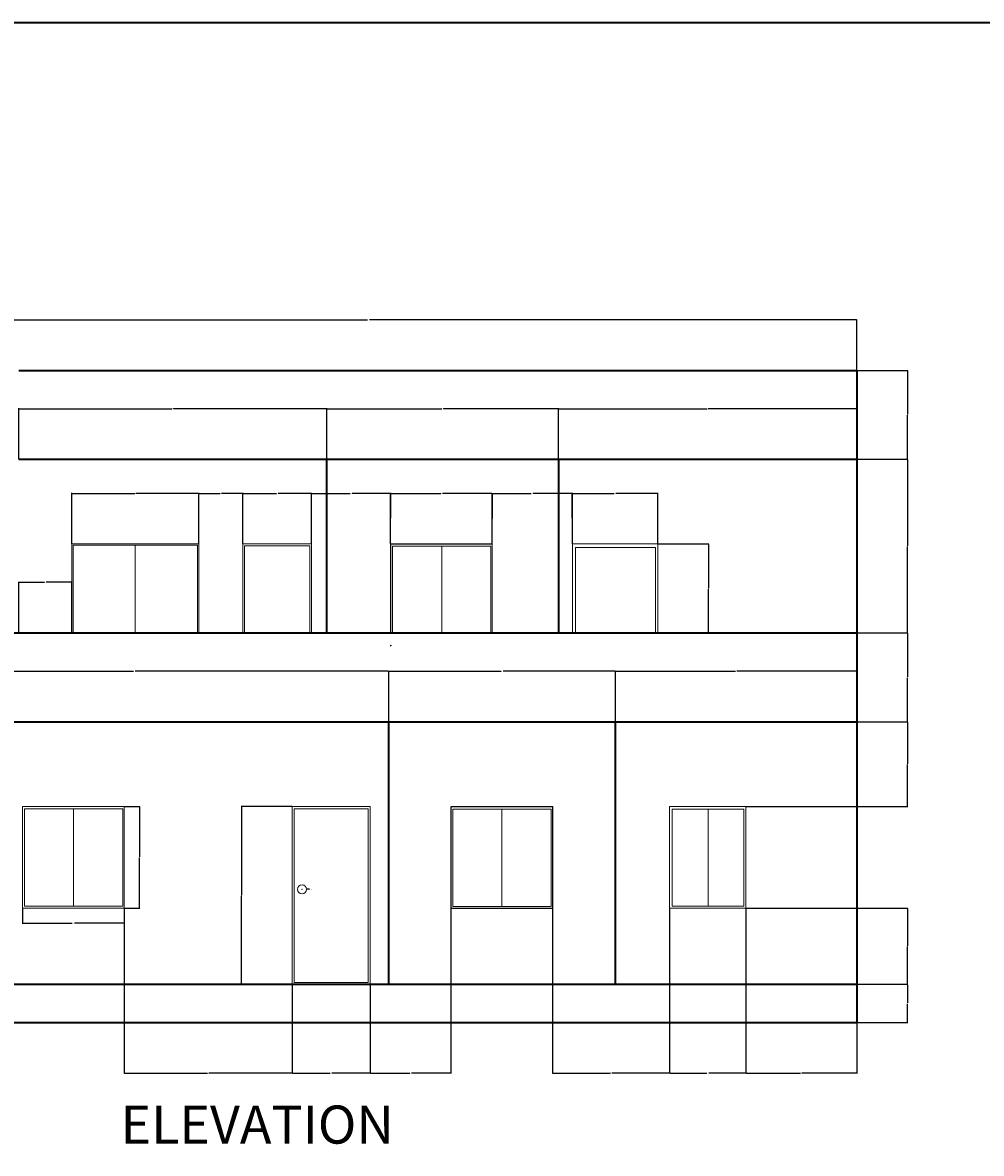
# Model space of a CAD drawing. Units: inches. Extents: x 2067 to 3463, y 1605 to 2723.
# Tile 7 of 10: x 2312 to 2765, y 2189 to 2723. Entities that reach past the tile are written whole.
import ezdxf

# ---------------------------------------------------------------- set-up
doc = ezdxf.new("R2010")
doc.units = ezdxf.units.IN
for name, color, linetype, lineweight in [('A-ANNO-DIMS', 2, 'Continuous', 18), ('A-ANNO-TEXT', 7, 'Continuous', 35), ('A-ANNO-TTLB', 7, 'Continuous', 35), ('A-ELEV', 7, 'Continuous', 35), ('A-ELEV-DOOR', 3, 'Continuous', 18), ('A-ELEV-GLAZ', 4, 'Continuous', 18)]:
    doc.layers.add(name, color=color, linetype=linetype, lineweight=lineweight)
doc.styles.get("Standard").update_dxf_attribs({"font": 'arial.ttf'})
doc.dimstyles.get("Standard").update_dxf_attribs({"dimtxt": 0.18, "dimasz": 0.18, "dimexe": 0.18, "dimexo": 0.0625, "dimgap": 0.09, "dimtad": 0, "dimtih": 1, "dimtoh": 1, "dimdec": 4, "dimzin": 0, "dimdsep": 46, "dimtxsty": 'Standard', "dimcen": 0.09, "dimadec": 0, "dimazin": 0, "dimtfac": 1, "dimtdec": 4, "dimtofl": 0, "dimtmove": 0, "dimatfit": 3, "dimfxl": 1, "dimtolj": 1, "dimtzin": 0, "dimarcsym": 0})

# ---------------------------------------------------------------- blocks, each defined once
blk = doc.blocks.new('WIN-ELEV-48X48')
for p, q in [((0, 48), (0, 0)), ((0, 48), (48, 48)), ((24.11, 0.97), (24.11, 46.96)), ((48, 48), (48, 0)), ((0, 0), (48, 0))]:
    blk.add_line(p, q)
blk.add_lwpolyline([(0.84, 46.96), (47.38, 46.96), (47.38, 0.97), (0.84, 0.97)], close=True)
blk = doc.blocks.new('*D26')
at = {"layer": 'A-ANNO-DIMS', "color": 0, "lineweight": -2, "transparency": 16777216}
for p, q in [((2360.32, 2352.37), (2367.64, 2352.37)), ((2367.46, 2352.19), (2367.46, 2328.55)), ((2367.46, 2304.55), (2367.46, 2328.18)), ((2360.32, 2304.37), (2367.64, 2304.37))]:
    blk.add_line(p, q, dxfattribs=at)
at = {"layer": 'A-ANNO-DIMS', "color": 0, "transparency": 16777216}
for points in [[(2367.43, 2352.19), (2367.49, 2352.19), (2367.46, 2352.37)], [(2367.43, 2304.55), (2367.49, 2304.55), (2367.46, 2304.37)]]:
    blk.add_solid(points, dxfattribs=at)
at = {"layer": 'Defpoints', "color": 0, "transparency": 16777216}
for p in [(2360.26, 2352.37), (2367.46, 2352.37), (2360.26, 2304.37)]:
    blk.add_point(p, dxfattribs=at)
at = {"layer": 'A-ANNO-DIMS', "color": 0, "transparency": 16777216, "insert": (2367.46, 2328.37), "char_height": 0.18, "attachment_point": 5}
blk.add_mtext('\\A1;WINDOW 48 TYP.', dxfattribs=at)
blk = doc.blocks.new('*D27')
at = {"layer": 'A-ANNO-DIMS', "color": 0, "lineweight": -2, "transparency": 16777216}
for p, q in [((2312.26, 2304.3), (2312.26, 2296.99)), ((2360.26, 2304.3), (2360.26, 2296.99)), ((2312.44, 2297.17), (2335.73, 2297.17)), ((2360.08, 2297.17), (2336.79, 2297.17))]:
    blk.add_line(p, q, dxfattribs=at)
at = {"layer": 'A-ANNO-DIMS', "color": 0, "transparency": 16777216}
for points in [[(2312.44, 2297.2), (2312.44, 2297.14), (2312.26, 2297.17)], [(2360.08, 2297.2), (2360.08, 2297.14), (2360.26, 2297.17)]]:
    blk.add_solid(points, dxfattribs=at)
at = {"layer": 'Defpoints', "color": 0, "transparency": 16777216}
for p in [(2312.26, 2304.37), (2360.26, 2304.37), (2360.26, 2297.17)]:
    blk.add_point(p, dxfattribs=at)
at = {"layer": 'A-ANNO-DIMS', "color": 0, "transparency": 16777216, "insert": (2336.26, 2297.17), "char_height": 0.18, "attachment_point": 5}
blk.add_mtext('\\A1;48 TYP.', dxfattribs=at)
blk = doc.blocks.new('*D69')
at = {"layer": 'A-ANNO-DIMS', "color": 0, "lineweight": -2, "transparency": 16777216}
for p, q in [((2244.95, 2434.43), (2244.95, 2582.45)), ((2245.13, 2582.27), (2475.3, 2582.27)), ((2706.27, 2582.27), (2476.1, 2582.27)), ((2706.45, 2558.43), (2706.45, 2582.45))]:
    blk.add_line(p, q, dxfattribs=at)
at = {"layer": 'A-ANNO-DIMS', "color": 0, "transparency": 16777216}
for points in [[(2245.13, 2582.3), (2245.13, 2582.24), (2244.95, 2582.27)], [(2706.27, 2582.3), (2706.27, 2582.24), (2706.45, 2582.27)]]:
    blk.add_solid(points, dxfattribs=at)
at = {"layer": 'Defpoints', "color": 0, "transparency": 16777216}
for p in [(2706.45, 2582.27), (2706.45, 2558.37), (2244.95, 2434.37)]:
    blk.add_point(p, dxfattribs=at)
at = {"layer": 'A-ANNO-DIMS', "color": 0, "transparency": 16777216, "insert": (2475.7, 2582.27), "char_height": 0.18, "attachment_point": 5}
blk.add_mtext('\\A1;461.5', dxfattribs=at)
blk = doc.blocks.new('*D71')
at = {"layer": 'A-ANNO-DIMS', "color": 0, "lineweight": -2, "transparency": 16777216}
for p, q in [((2706.51, 2268.37), (2730.53, 2268.37)), ((2730.35, 2268.19), (2730.35, 2259.55)), ((2730.35, 2250.55), (2730.35, 2259.18)), ((2706.51, 2250.37), (2730.53, 2250.37))]:
    blk.add_line(p, q, dxfattribs=at)
at = {"layer": 'A-ANNO-DIMS', "color": 0, "transparency": 16777216}
for points in [[(2730.32, 2268.19), (2730.38, 2268.19), (2730.35, 2268.37)], [(2730.32, 2250.55), (2730.38, 2250.55), (2730.35, 2250.37)]]:
    blk.add_solid(points, dxfattribs=at)
at = {"layer": 'Defpoints', "color": 0, "transparency": 16777216}
for p in [(2706.45, 2268.37), (2730.35, 2268.37), (2706.45, 2250.37)]:
    blk.add_point(p, dxfattribs=at)
at = {"layer": 'A-ANNO-DIMS', "color": 0, "transparency": 16777216, "insert": (2730.35, 2259.37), "char_height": 0.18, "attachment_point": 5}
blk.add_mtext('\\A1;18', dxfattribs=at)
blk = doc.blocks.new('*D72')
at = {"layer": 'A-ANNO-DIMS', "color": 0, "lineweight": -2, "transparency": 16777216}
for p, q in [((2654.01, 2304.37), (2730.53, 2304.37)), ((2730.35, 2304.19), (2730.35, 2286.55)), ((2730.35, 2268.55), (2730.35, 2286.18)), ((2706.51, 2268.37), (2730.53, 2268.37))]:
    blk.add_line(p, q, dxfattribs=at)
at = {"layer": 'A-ANNO-DIMS', "color": 0, "transparency": 16777216}
for points in [[(2730.32, 2304.19), (2730.38, 2304.19), (2730.35, 2304.37)], [(2730.32, 2268.55), (2730.38, 2268.55), (2730.35, 2268.37)]]:
    blk.add_solid(points, dxfattribs=at)
at = {"layer": 'Defpoints', "color": 0, "transparency": 16777216}
for p in [(2653.95, 2304.37), (2730.35, 2304.37), (2706.45, 2268.37)]:
    blk.add_point(p, dxfattribs=at)
at = {"layer": 'A-ANNO-DIMS', "color": 0, "transparency": 16777216, "insert": (2730.35, 2286.37), "char_height": 0.18, "attachment_point": 5}
blk.add_mtext('\\A1;36', dxfattribs=at)
blk = doc.blocks.new('*D73')
at = {"layer": 'A-ANNO-DIMS', "color": 0, "lineweight": -2, "transparency": 16777216}
for p, q in [((2706.51, 2392.37), (2730.53, 2392.37)), ((2730.35, 2392.19), (2730.35, 2372.55)), ((2730.35, 2352.55), (2730.35, 2372.18)), ((2654.01, 2352.37), (2730.53, 2352.37))]:
    blk.add_line(p, q, dxfattribs=at)
at = {"layer": 'A-ANNO-DIMS', "color": 0, "transparency": 16777216}
for points in [[(2730.32, 2392.19), (2730.38, 2392.19), (2730.35, 2392.37)], [(2730.32, 2352.55), (2730.38, 2352.55), (2730.35, 2352.37)]]:
    blk.add_solid(points, dxfattribs=at)
at = {"layer": 'Defpoints', "color": 0, "transparency": 16777216}
for p in [(2706.45, 2392.37), (2730.35, 2392.37), (2653.95, 2352.37)]:
    blk.add_point(p, dxfattribs=at)
at = {"layer": 'A-ANNO-DIMS', "color": 0, "transparency": 16777216, "insert": (2730.35, 2372.37), "char_height": 0.18, "attachment_point": 5}
blk.add_mtext('\\A1;40', dxfattribs=at)
blk = doc.blocks.new('*D74')
at = {"layer": 'A-ANNO-DIMS', "color": 0, "lineweight": -2, "transparency": 16777216}
for p, q in [((2706.51, 2434.37), (2730.53, 2434.37)), ((2730.35, 2434.19), (2730.35, 2413.55)), ((2730.35, 2392.55), (2730.35, 2413.19)), ((2706.51, 2392.37), (2730.53, 2392.37))]:
    blk.add_line(p, q, dxfattribs=at)
at = {"layer": 'A-ANNO-DIMS', "color": 0, "transparency": 16777216}
for points in [[(2730.32, 2434.19), (2730.38, 2434.19), (2730.35, 2434.37)], [(2730.32, 2392.55), (2730.38, 2392.55), (2730.35, 2392.37)]]:
    blk.add_solid(points, dxfattribs=at)
at = {"layer": 'Defpoints', "color": 0, "transparency": 16777216}
for p in [(2706.45, 2434.37), (2730.35, 2434.37), (2706.45, 2392.37)]:
    blk.add_point(p, dxfattribs=at)
at = {"layer": 'A-ANNO-DIMS', "color": 0, "transparency": 16777216, "insert": (2730.35, 2413.37), "char_height": 0.18, "attachment_point": 5}
blk.add_mtext('\\A1;42', dxfattribs=at)
blk = doc.blocks.new('*D75')
at = {"layer": 'A-ANNO-DIMS', "color": 0, "lineweight": -2, "transparency": 16777216}
for p, q in [((2706.51, 2516.37), (2730.53, 2516.37)), ((2730.35, 2516.19), (2730.35, 2475.55)), ((2730.35, 2434.55), (2730.35, 2475.18)), ((2706.51, 2434.37), (2730.53, 2434.37))]:
    blk.add_line(p, q, dxfattribs=at)
at = {"layer": 'A-ANNO-DIMS', "color": 0, "transparency": 16777216}
for points in [[(2730.32, 2516.19), (2730.38, 2516.19), (2730.35, 2516.37)], [(2730.32, 2434.55), (2730.38, 2434.55), (2730.35, 2434.37)]]:
    blk.add_solid(points, dxfattribs=at)
at = {"layer": 'Defpoints', "color": 0, "transparency": 16777216}
for p in [(2706.45, 2516.37), (2730.35, 2516.37), (2706.45, 2434.37)]:
    blk.add_point(p, dxfattribs=at)
at = {"layer": 'A-ANNO-DIMS', "color": 0, "transparency": 16777216, "insert": (2730.35, 2475.37), "char_height": 0.18, "attachment_point": 5}
blk.add_mtext('\\A1;82', dxfattribs=at)
blk = doc.blocks.new('*D76')
at = {"layer": 'A-ANNO-DIMS', "color": 0, "lineweight": -2, "transparency": 16777216}
for p, q in [((2706.51, 2558.37), (2730.53, 2558.37)), ((2730.35, 2558.19), (2730.35, 2537.55)), ((2730.35, 2516.55), (2730.35, 2537.19)), ((2706.51, 2516.37), (2730.53, 2516.37))]:
    blk.add_line(p, q, dxfattribs=at)
at = {"layer": 'A-ANNO-DIMS', "color": 0, "transparency": 16777216}
for points in [[(2730.32, 2558.19), (2730.38, 2558.19), (2730.35, 2558.37)], [(2730.32, 2516.55), (2730.38, 2516.55), (2730.35, 2516.37)]]:
    blk.add_solid(points, dxfattribs=at)
at = {"layer": 'Defpoints', "color": 0, "transparency": 16777216}
for p in [(2706.45, 2558.37), (2730.35, 2558.37), (2706.45, 2516.37)]:
    blk.add_point(p, dxfattribs=at)
at = {"layer": 'A-ANNO-DIMS', "color": 0, "transparency": 16777216, "insert": (2730.35, 2537.37), "char_height": 0.18, "attachment_point": 5}
blk.add_mtext('\\A1;42', dxfattribs=at)
blk = doc.blocks.new('*D78')
at = {"layer": 'A-ANNO-DIMS', "color": 0, "lineweight": -2, "transparency": 16777216}
for p, q in [((2310.45, 2516.43), (2310.45, 2540.45)), ((2310.63, 2540.27), (2382.81, 2540.27)), ((2455.77, 2540.27), (2383.58, 2540.27)), ((2455.95, 2516.43), (2455.95, 2540.45))]:
    blk.add_line(p, q, dxfattribs=at)
at = {"layer": 'A-ANNO-DIMS', "color": 0, "transparency": 16777216}
for points in [[(2310.63, 2540.3), (2310.63, 2540.24), (2310.45, 2540.27)], [(2455.77, 2540.3), (2455.77, 2540.24), (2455.95, 2540.27)]]:
    blk.add_solid(points, dxfattribs=at)
at = {"layer": 'Defpoints', "color": 0, "transparency": 16777216}
for p in [(2455.95, 2540.27), (2310.45, 2516.37), (2455.95, 2516.37)]:
    blk.add_point(p, dxfattribs=at)
at = {"layer": 'A-ANNO-DIMS', "color": 0, "transparency": 16777216, "insert": (2383.2, 2540.27), "char_height": 0.18, "attachment_point": 5}
blk.add_mtext('\\A1;145.5', dxfattribs=at)
blk = doc.blocks.new('*D79')
at = {"layer": 'A-ANNO-DIMS', "color": 0, "lineweight": -2, "transparency": 16777216}
for p, q in [((2455.95, 2516.43), (2455.95, 2540.45)), ((2456.13, 2540.27), (2510.31, 2540.27)), ((2565.27, 2540.27), (2511.08, 2540.27)), ((2565.45, 2516.43), (2565.45, 2540.45))]:
    blk.add_line(p, q, dxfattribs=at)
at = {"layer": 'A-ANNO-DIMS', "color": 0, "transparency": 16777216}
for points in [[(2456.13, 2540.3), (2456.13, 2540.24), (2455.95, 2540.27)], [(2565.27, 2540.3), (2565.27, 2540.24), (2565.45, 2540.27)]]:
    blk.add_solid(points, dxfattribs=at)
at = {"layer": 'Defpoints', "color": 0, "transparency": 16777216}
for p in [(2565.45, 2540.27), (2455.95, 2516.37), (2565.45, 2516.37)]:
    blk.add_point(p, dxfattribs=at)
at = {"layer": 'A-ANNO-DIMS', "color": 0, "transparency": 16777216, "insert": (2510.7, 2540.27), "char_height": 0.18, "attachment_point": 5}
blk.add_mtext('\\A1;109.5', dxfattribs=at)
blk = doc.blocks.new('*D80')
at = {"layer": 'A-ANNO-DIMS', "color": 0, "lineweight": -2, "transparency": 16777216}
for p, q in [((2565.45, 2516.43), (2565.45, 2540.45)), ((2565.63, 2540.27), (2635.68, 2540.27)), ((2706.27, 2540.27), (2636.21, 2540.27)), ((2706.45, 2516.43), (2706.45, 2540.45))]:
    blk.add_line(p, q, dxfattribs=at)
at = {"layer": 'A-ANNO-DIMS', "color": 0, "transparency": 16777216}
for points in [[(2565.63, 2540.3), (2565.63, 2540.24), (2565.45, 2540.27)], [(2706.27, 2540.3), (2706.27, 2540.24), (2706.45, 2540.27)]]:
    blk.add_solid(points, dxfattribs=at)
at = {"layer": 'Defpoints', "color": 0, "transparency": 16777216}
for p in [(2706.45, 2540.27), (2565.45, 2516.37), (2706.45, 2516.37)]:
    blk.add_point(p, dxfattribs=at)
at = {"layer": 'A-ANNO-DIMS', "color": 0, "transparency": 16777216, "insert": (2635.95, 2540.27), "char_height": 0.18, "attachment_point": 5}
blk.add_mtext('\\A1;141', dxfattribs=at)
blk = doc.blocks.new('*D81')
at = {"layer": 'A-ANNO-DIMS', "color": 0, "lineweight": -2, "transparency": 16777216}
for p, q in [((2310.45, 2434.43), (2310.45, 2458.45)), ((2310.63, 2458.27), (2322.63, 2458.27)), ((2335.38, 2458.27), (2323.38, 2458.27)), ((2335.56, 2434.43), (2335.56, 2458.45))]:
    blk.add_line(p, q, dxfattribs=at)
at = {"layer": 'A-ANNO-DIMS', "color": 0, "transparency": 16777216}
for points in [[(2310.63, 2458.3), (2310.63, 2458.24), (2310.45, 2458.27)], [(2335.38, 2458.3), (2335.38, 2458.24), (2335.56, 2458.27)]]:
    blk.add_solid(points, dxfattribs=at)
at = {"layer": 'Defpoints', "color": 0, "transparency": 16777216}
for p in [(2335.56, 2458.27), (2310.45, 2434.37), (2335.56, 2434.37)]:
    blk.add_point(p, dxfattribs=at)
at = {"layer": 'A-ANNO-DIMS', "color": 0, "transparency": 16777216, "insert": (2323, 2458.27), "char_height": 0.18, "attachment_point": 5}
blk.add_mtext('\\A1;25.11', dxfattribs=at)
blk = doc.blocks.new('*D82')
at = {"layer": 'A-ANNO-DIMS', "color": 0, "lineweight": -2, "transparency": 16777216}
for p, q in [((2335.56, 2476.43), (2335.56, 2500.45)), ((2335.74, 2500.27), (2365.34, 2500.27)), ((2395.38, 2500.27), (2365.78, 2500.27)), ((2395.56, 2476.43), (2395.56, 2500.45))]:
    blk.add_line(p, q, dxfattribs=at)
at = {"layer": 'A-ANNO-DIMS', "color": 0, "transparency": 16777216}
for points in [[(2335.74, 2500.3), (2335.74, 2500.24), (2335.56, 2500.27)], [(2395.38, 2500.3), (2395.38, 2500.24), (2395.56, 2500.27)]]:
    blk.add_solid(points, dxfattribs=at)
at = {"layer": 'Defpoints', "color": 0, "transparency": 16777216}
for p in [(2395.56, 2500.27), (2335.56, 2476.37), (2395.56, 2476.37)]:
    blk.add_point(p, dxfattribs=at)
at = {"layer": 'A-ANNO-DIMS', "color": 0, "transparency": 16777216, "insert": (2365.56, 2500.27), "char_height": 0.18, "attachment_point": 5}
blk.add_mtext('\\A1;60', dxfattribs=at)
blk = doc.blocks.new('*D83')
at = {"layer": 'A-ANNO-DIMS', "color": 0, "lineweight": -2, "transparency": 16777216}
for p, q in [((2395.56, 2476.43), (2395.56, 2500.45)), ((2395.74, 2500.27), (2405.63, 2500.27)), ((2416.18, 2500.27), (2406.28, 2500.27)), ((2416.36, 2476.43), (2416.36, 2500.45))]:
    blk.add_line(p, q, dxfattribs=at)
at = {"layer": 'A-ANNO-DIMS', "color": 0, "transparency": 16777216}
for points in [[(2395.74, 2500.3), (2395.74, 2500.24), (2395.56, 2500.27)], [(2416.18, 2500.3), (2416.18, 2500.24), (2416.36, 2500.27)]]:
    blk.add_solid(points, dxfattribs=at)
at = {"layer": 'Defpoints', "color": 0, "transparency": 16777216}
for p in [(2416.36, 2500.27), (2395.56, 2476.37), (2416.36, 2476.37)]:
    blk.add_point(p, dxfattribs=at)
at = {"layer": 'A-ANNO-DIMS', "color": 0, "transparency": 16777216, "insert": (2405.96, 2500.27), "char_height": 0.18, "attachment_point": 5}
blk.add_mtext('\\A1;20.8', dxfattribs=at)
blk = doc.blocks.new('*D84')
at = {"layer": 'A-ANNO-DIMS', "color": 0, "lineweight": -2, "transparency": 16777216}
for p, q in [((2416.36, 2476.43), (2416.36, 2500.45)), ((2416.54, 2500.27), (2432.18, 2500.27)), ((2448.62, 2500.27), (2432.97, 2500.27)), ((2448.8, 2476.43), (2448.8, 2500.45))]:
    blk.add_line(p, q, dxfattribs=at)
at = {"layer": 'A-ANNO-DIMS', "color": 0, "transparency": 16777216}
for points in [[(2416.54, 2500.3), (2416.54, 2500.24), (2416.36, 2500.27)], [(2448.62, 2500.3), (2448.62, 2500.24), (2448.8, 2500.27)]]:
    blk.add_solid(points, dxfattribs=at)
at = {"layer": 'Defpoints', "color": 0, "transparency": 16777216}
for p in [(2448.8, 2500.27), (2416.36, 2476.37), (2448.8, 2476.37)]:
    blk.add_point(p, dxfattribs=at)
at = {"layer": 'A-ANNO-DIMS', "color": 0, "transparency": 16777216, "insert": (2432.58, 2500.27), "char_height": 0.18, "attachment_point": 5}
blk.add_mtext('\\A1;32.44', dxfattribs=at)
blk = doc.blocks.new('*D85')
at = {"layer": 'A-ANNO-DIMS', "color": 0, "lineweight": -2, "transparency": 16777216}
for p, q in [((2448.8, 2476.43), (2448.8, 2500.45)), ((2448.98, 2500.27), (2467.02, 2500.27)), ((2485.98, 2500.27), (2467.94, 2500.27)), ((2486.16, 2476.43), (2486.16, 2500.45))]:
    blk.add_line(p, q, dxfattribs=at)
at = {"layer": 'A-ANNO-DIMS', "color": 0, "transparency": 16777216}
for points in [[(2448.98, 2500.3), (2448.98, 2500.24), (2448.8, 2500.27)], [(2485.98, 2500.3), (2485.98, 2500.24), (2486.16, 2500.27)]]:
    blk.add_solid(points, dxfattribs=at)
at = {"layer": 'Defpoints', "color": 0, "transparency": 16777216}
for p in [(2486.16, 2500.27), (2448.8, 2476.37), (2486.16, 2476.37)]:
    blk.add_point(p, dxfattribs=at)
at = {"layer": 'A-ANNO-DIMS', "color": 0, "transparency": 16777216, "insert": (2467.48, 2500.27), "char_height": 0.18, "attachment_point": 5}
blk.add_mtext('\\A1;37.365', dxfattribs=at)
blk = doc.blocks.new('*D86')
at = {"layer": 'A-ANNO-DIMS', "color": 0, "lineweight": -2, "transparency": 16777216}
for p, q in [((2486.16, 2476.43), (2486.2, 2500.45)), ((2486.38, 2500.27), (2509.81, 2500.23)), ((2534.04, 2500.19), (2510.61, 2500.23)), ((2534.18, 2476.35), (2534.22, 2500.37))]:
    blk.add_line(p, q, dxfattribs=at)
at = {"layer": 'A-ANNO-DIMS', "color": 0, "transparency": 16777216}
for points in [[(2486.38, 2500.3), (2486.38, 2500.24), (2486.2, 2500.27)], [(2534.04, 2500.22), (2534.04, 2500.16), (2534.22, 2500.19)]]:
    blk.add_solid(points, dxfattribs=at)
at = {"layer": 'Defpoints', "color": 0, "transparency": 16777216}
for p in [(2534.22, 2500.19), (2486.16, 2476.37), (2534.18, 2476.29)]:
    blk.add_point(p, dxfattribs=at)
at = {"layer": 'A-ANNO-DIMS', "color": 0, "transparency": 16777216, "insert": (2510.21, 2500.23), "char_height": 0.18, "attachment_point": 5}
blk.add_mtext('\\A1;48.02', dxfattribs=at)
blk = doc.blocks.new('*D87')
at = {"layer": 'A-ANNO-DIMS', "color": 0, "lineweight": -2, "transparency": 16777216}
for p, q in [((2534.18, 2476.35), (2534.14, 2500.37)), ((2534.32, 2500.19), (2552.59, 2500.23)), ((2571.8, 2500.27), (2553.52, 2500.23)), ((2572.03, 2476.43), (2571.98, 2500.45))]:
    blk.add_line(p, q, dxfattribs=at)
at = {"layer": 'A-ANNO-DIMS', "color": 0, "transparency": 16777216}
for points in [[(2534.32, 2500.22), (2534.32, 2500.16), (2534.14, 2500.19)], [(2571.8, 2500.3), (2571.8, 2500.24), (2571.98, 2500.27)]]:
    blk.add_solid(points, dxfattribs=at)
at = {"layer": 'Defpoints', "color": 0, "transparency": 16777216}
for p in [(2571.98, 2500.27), (2534.18, 2476.29), (2572.03, 2476.37)]:
    blk.add_point(p, dxfattribs=at)
at = {"layer": 'A-ANNO-DIMS', "color": 0, "transparency": 16777216, "insert": (2553.06, 2500.23), "char_height": 0.18, "attachment_point": 5}
blk.add_mtext('\\A1;37.844', dxfattribs=at)
blk = doc.blocks.new('*D88')
at = {"layer": 'A-ANNO-DIMS', "color": 0, "lineweight": -2, "transparency": 16777216}
for p, q in [((2572.03, 2476.43), (2572.03, 2500.45)), ((2572.21, 2500.27), (2591.84, 2500.27)), ((2612.27, 2500.27), (2592.63, 2500.27)), ((2612.45, 2476.43), (2612.45, 2500.45))]:
    blk.add_line(p, q, dxfattribs=at)
at = {"layer": 'A-ANNO-DIMS', "color": 0, "transparency": 16777216}
for points in [[(2572.21, 2500.3), (2572.21, 2500.24), (2572.03, 2500.27)], [(2612.27, 2500.3), (2612.27, 2500.24), (2612.45, 2500.27)]]:
    blk.add_solid(points, dxfattribs=at)
at = {"layer": 'Defpoints', "color": 0, "transparency": 16777216}
for p in [(2612.45, 2500.27), (2572.03, 2476.37), (2612.45, 2476.37)]:
    blk.add_point(p, dxfattribs=at)
at = {"layer": 'A-ANNO-DIMS', "color": 0, "transparency": 16777216, "insert": (2592.24, 2500.27), "char_height": 0.18, "attachment_point": 5}
blk.add_mtext('\\A1;40.42', dxfattribs=at)
blk = doc.blocks.new('*D89')
at = {"layer": 'A-ANNO-DIMS', "color": 0, "lineweight": -2, "transparency": 16777216}
for p, q in [((2612.51, 2476.37), (2636.53, 2476.37)), ((2636.35, 2476.19), (2636.35, 2455.55)), ((2636.35, 2434.55), (2636.35, 2455.19)), ((2612.51, 2434.37), (2636.53, 2434.37))]:
    blk.add_line(p, q, dxfattribs=at)
at = {"layer": 'A-ANNO-DIMS', "color": 0, "transparency": 16777216}
for points in [[(2636.32, 2476.19), (2636.38, 2476.19), (2636.35, 2476.37)], [(2636.32, 2434.55), (2636.38, 2434.55), (2636.35, 2434.37)]]:
    blk.add_solid(points, dxfattribs=at)
at = {"layer": 'Defpoints', "color": 0, "transparency": 16777216}
for p in [(2612.45, 2476.37), (2612.45, 2434.37), (2636.35, 2434.37)]:
    blk.add_point(p, dxfattribs=at)
at = {"layer": 'A-ANNO-DIMS', "color": 0, "transparency": 16777216, "insert": (2636.35, 2455.37), "char_height": 0.18, "attachment_point": 5}
blk.add_mtext('\\A1;42', dxfattribs=at)
blk = doc.blocks.new('*D92')
at = {"layer": 'A-ANNO-DIMS', "color": 0, "lineweight": -2, "transparency": 16777216}
for p, q in [((2360.26, 2304.3), (2360.26, 2226.29)), ((2439.62, 2268.3), (2439.62, 2226.29)), ((2360.44, 2226.47), (2399.55, 2226.47)), ((2439.44, 2226.47), (2400.33, 2226.47))]:
    blk.add_line(p, q, dxfattribs=at)
at = {"layer": 'A-ANNO-DIMS', "color": 0, "transparency": 16777216}
for points in [[(2360.44, 2226.5), (2360.44, 2226.44), (2360.26, 2226.47)], [(2439.44, 2226.5), (2439.44, 2226.44), (2439.62, 2226.47)]]:
    blk.add_solid(points, dxfattribs=at)
at = {"layer": 'Defpoints', "color": 0, "transparency": 16777216}
for p in [(2360.26, 2304.37), (2439.62, 2268.37), (2439.62, 2226.47)]:
    blk.add_point(p, dxfattribs=at)
at = {"layer": 'A-ANNO-DIMS', "color": 0, "transparency": 16777216, "insert": (2399.94, 2226.47), "char_height": 0.18, "attachment_point": 5}
blk.add_mtext('\\A1;79.36', dxfattribs=at)
blk = doc.blocks.new('*D93')
at = {"layer": 'A-ANNO-DIMS', "color": 0, "lineweight": -2, "transparency": 16777216}
for p, q in [((2439.62, 2268.3), (2439.62, 2226.29)), ((2476.48, 2268.3), (2476.48, 2226.29)), ((2439.8, 2226.47), (2457.66, 2226.47)), ((2476.3, 2226.47), (2458.44, 2226.47))]:
    blk.add_line(p, q, dxfattribs=at)
at = {"layer": 'A-ANNO-DIMS', "color": 0, "transparency": 16777216}
for points in [[(2439.8, 2226.5), (2439.8, 2226.44), (2439.62, 2226.47)], [(2476.3, 2226.5), (2476.3, 2226.44), (2476.48, 2226.47)]]:
    blk.add_solid(points, dxfattribs=at)
at = {"layer": 'Defpoints', "color": 0, "transparency": 16777216}
for p in [(2439.62, 2268.37), (2476.48, 2268.37), (2476.48, 2226.47)]:
    blk.add_point(p, dxfattribs=at)
at = {"layer": 'A-ANNO-DIMS', "color": 0, "transparency": 16777216, "insert": (2458.05, 2226.47), "char_height": 0.18, "attachment_point": 5}
blk.add_mtext('\\A1;36.86', dxfattribs=at)
blk = doc.blocks.new('*D94')
at = {"layer": 'A-ANNO-DIMS', "color": 0, "lineweight": -2, "transparency": 16777216}
for p, q in [((2514.64, 2304.14), (2514.64, 2226.29)), ((2476.48, 2268.3), (2476.48, 2226.29)), ((2476.66, 2226.47), (2495.17, 2226.47)), ((2514.46, 2226.47), (2495.95, 2226.47))]:
    blk.add_line(p, q, dxfattribs=at)
at = {"layer": 'A-ANNO-DIMS', "color": 0, "transparency": 16777216}
for points in [[(2476.66, 2226.5), (2476.66, 2226.44), (2476.48, 2226.47)], [(2514.46, 2226.5), (2514.46, 2226.44), (2514.64, 2226.47)]]:
    blk.add_solid(points, dxfattribs=at)
at = {"layer": 'Defpoints', "color": 0, "transparency": 16777216}
for p in [(2514.64, 2304.2), (2476.48, 2268.37), (2514.64, 2226.47)]:
    blk.add_point(p, dxfattribs=at)
at = {"layer": 'A-ANNO-DIMS', "color": 0, "transparency": 16777216, "insert": (2495.56, 2226.47), "char_height": 0.18, "attachment_point": 5}
blk.add_mtext('\\A1;38.16', dxfattribs=at)
blk = doc.blocks.new('*D95')
at = {"layer": 'A-ANNO-DIMS', "color": 0, "lineweight": -2, "transparency": 16777216}
for p, q in [((2562.64, 2304.14), (2562.64, 2226.29)), ((2617.98, 2304.3), (2617.98, 2226.29)), ((2562.82, 2226.47), (2589.92, 2226.47)), ((2617.8, 2226.47), (2590.7, 2226.47))]:
    blk.add_line(p, q, dxfattribs=at)
at = {"layer": 'A-ANNO-DIMS', "color": 0, "transparency": 16777216}
for points in [[(2562.82, 2226.5), (2562.82, 2226.44), (2562.64, 2226.47)], [(2617.8, 2226.5), (2617.8, 2226.44), (2617.98, 2226.47)]]:
    blk.add_solid(points, dxfattribs=at)
at = {"layer": 'Defpoints', "color": 0, "transparency": 16777216}
for p in [(2562.64, 2304.2), (2617.98, 2304.37), (2617.98, 2226.47)]:
    blk.add_point(p, dxfattribs=at)
at = {"layer": 'A-ANNO-DIMS', "color": 0, "transparency": 16777216, "insert": (2590.31, 2226.47), "char_height": 0.18, "attachment_point": 5}
blk.add_mtext('\\A1;55.34', dxfattribs=at)
blk = doc.blocks.new('*D96')
at = {"layer": 'A-ANNO-DIMS', "color": 0, "lineweight": -2, "transparency": 16777216}
for p, q in [((2617.98, 2304.3), (2617.98, 2226.29)), ((2653.95, 2304.3), (2653.95, 2226.29)), ((2618.16, 2226.47), (2635.5, 2226.47)), ((2653.77, 2226.47), (2636.43, 2226.47))]:
    blk.add_line(p, q, dxfattribs=at)
at = {"layer": 'A-ANNO-DIMS', "color": 0, "transparency": 16777216}
for points in [[(2618.16, 2226.5), (2618.16, 2226.44), (2617.98, 2226.47)], [(2653.77, 2226.5), (2653.77, 2226.44), (2653.95, 2226.47)]]:
    blk.add_solid(points, dxfattribs=at)
at = {"layer": 'Defpoints', "color": 0, "transparency": 16777216}
for p in [(2617.98, 2304.37), (2653.95, 2304.37), (2653.95, 2226.47)]:
    blk.add_point(p, dxfattribs=at)
at = {"layer": 'A-ANNO-DIMS', "color": 0, "transparency": 16777216, "insert": (2635.96, 2226.47), "char_height": 0.18, "attachment_point": 5}
blk.add_mtext('\\A1;35.966', dxfattribs=at)
blk = doc.blocks.new('*D97')
at = {"layer": 'A-ANNO-DIMS', "color": 0, "lineweight": -2, "transparency": 16777216}
for p, q in [((2653.95, 2304.3), (2653.95, 2226.29)), ((2706.45, 2250.3), (2706.45, 2226.29)), ((2654.13, 2226.47), (2679.87, 2226.47)), ((2706.27, 2226.47), (2680.52, 2226.47))]:
    blk.add_line(p, q, dxfattribs=at)
at = {"layer": 'A-ANNO-DIMS', "color": 0, "transparency": 16777216}
for points in [[(2654.13, 2226.5), (2654.13, 2226.44), (2653.95, 2226.47)], [(2706.27, 2226.5), (2706.27, 2226.44), (2706.45, 2226.47)]]:
    blk.add_solid(points, dxfattribs=at)
at = {"layer": 'Defpoints', "color": 0, "transparency": 16777216}
for p in [(2653.95, 2304.37), (2706.45, 2250.37), (2706.45, 2226.47)]:
    blk.add_point(p, dxfattribs=at)
at = {"layer": 'A-ANNO-DIMS', "color": 0, "transparency": 16777216, "insert": (2680.2, 2226.47), "char_height": 0.18, "attachment_point": 5}
blk.add_mtext('\\A1;52.5', dxfattribs=at)
blk = doc.blocks.new('*D98')
at = {"layer": 'A-ANNO-DIMS', "color": 0, "lineweight": -2, "transparency": 16777216}
for p, q in [((2439.56, 2352.37), (2415.54, 2352.37)), ((2415.72, 2352.19), (2415.72, 2310.55)), ((2415.72, 2268.55), (2415.72, 2310.18)), ((2439.56, 2268.37), (2415.54, 2268.37))]:
    blk.add_line(p, q, dxfattribs=at)
at = {"layer": 'A-ANNO-DIMS', "color": 0, "transparency": 16777216}
for points in [[(2415.69, 2352.19), (2415.75, 2352.19), (2415.72, 2352.37)], [(2415.69, 2268.55), (2415.75, 2268.55), (2415.72, 2268.37)]]:
    blk.add_solid(points, dxfattribs=at)
at = {"layer": 'Defpoints', "color": 0, "transparency": 16777216}
for p in [(2415.72, 2352.37), (2439.62, 2352.37), (2439.62, 2268.37)]:
    blk.add_point(p, dxfattribs=at)
at = {"layer": 'A-ANNO-DIMS', "color": 0, "transparency": 16777216, "insert": (2415.72, 2310.37), "char_height": 0.18, "attachment_point": 5}
blk.add_mtext('\\A1;84', dxfattribs=at)
blk = doc.blocks.new('*D99')
at = {"layer": 'A-ANNO-DIMS', "color": 0, "lineweight": -2, "transparency": 16777216}
for p, q in [((2244.95, 2392.43), (2244.95, 2416.45)), ((2245.13, 2416.27), (2364.7, 2416.27)), ((2485.06, 2416.27), (2365.49, 2416.27)), ((2485.24, 2392.43), (2485.24, 2416.45))]:
    blk.add_line(p, q, dxfattribs=at)
at = {"layer": 'A-ANNO-DIMS', "color": 0, "transparency": 16777216}
for points in [[(2245.13, 2416.3), (2245.13, 2416.24), (2244.95, 2416.27)], [(2485.06, 2416.3), (2485.06, 2416.24), (2485.24, 2416.27)]]:
    blk.add_solid(points, dxfattribs=at)
at = {"layer": 'Defpoints', "color": 0, "transparency": 16777216}
for p in [(2485.24, 2416.27), (2244.95, 2392.37), (2485.24, 2392.37)]:
    blk.add_point(p, dxfattribs=at)
at = {"layer": 'A-ANNO-DIMS', "color": 0, "transparency": 16777216, "insert": (2365.09, 2416.27), "char_height": 0.18, "attachment_point": 5}
blk.add_mtext('\\A1;240.3', dxfattribs=at)
blk = doc.blocks.new('*D100')
at = {"layer": 'A-ANNO-DIMS', "color": 0, "lineweight": -2, "transparency": 16777216}
for p, q in [((2485.24, 2392.43), (2485.24, 2416.45)), ((2485.42, 2416.27), (2538.4, 2416.27)), ((2592.27, 2416.27), (2539.28, 2416.27)), ((2592.45, 2392.43), (2592.45, 2416.45))]:
    blk.add_line(p, q, dxfattribs=at)
at = {"layer": 'A-ANNO-DIMS', "color": 0, "transparency": 16777216}
for points in [[(2485.42, 2416.3), (2485.42, 2416.24), (2485.24, 2416.27)], [(2592.27, 2416.3), (2592.27, 2416.24), (2592.45, 2416.27)]]:
    blk.add_solid(points, dxfattribs=at)
at = {"layer": 'Defpoints', "color": 0, "transparency": 16777216}
for p in [(2592.45, 2416.27), (2485.24, 2392.37), (2592.45, 2392.37)]:
    blk.add_point(p, dxfattribs=at)
at = {"layer": 'A-ANNO-DIMS', "color": 0, "transparency": 16777216, "insert": (2538.84, 2416.27), "char_height": 0.18, "attachment_point": 5}
blk.add_mtext('\\A1;107.21', dxfattribs=at)
blk = doc.blocks.new('*D101')
at = {"layer": 'A-ANNO-DIMS', "color": 0, "lineweight": -2, "transparency": 16777216}
for p, q in [((2592.45, 2392.43), (2592.45, 2416.45)), ((2592.63, 2416.27), (2649.17, 2416.27)), ((2706.27, 2416.27), (2649.73, 2416.27)), ((2706.45, 2392.43), (2706.45, 2416.45))]:
    blk.add_line(p, q, dxfattribs=at)
at = {"layer": 'A-ANNO-DIMS', "color": 0, "transparency": 16777216}
for points in [[(2592.63, 2416.3), (2592.63, 2416.24), (2592.45, 2416.27)], [(2706.27, 2416.3), (2706.27, 2416.24), (2706.45, 2416.27)]]:
    blk.add_solid(points, dxfattribs=at)
at = {"layer": 'Defpoints', "color": 0, "transparency": 16777216}
for p in [(2706.45, 2416.27), (2592.45, 2392.37), (2706.45, 2392.37)]:
    blk.add_point(p, dxfattribs=at)
at = {"layer": 'A-ANNO-DIMS', "color": 0, "transparency": 16777216, "insert": (2649.45, 2416.27), "char_height": 0.18, "attachment_point": 5}
blk.add_mtext('\\A1;114', dxfattribs=at)
blk = doc.blocks.new('*D115')
at = {"layer": 'A-ANNO-DIMS', "color": 0, "lineweight": -2, "transparency": 16777216}
for p, q in [((2444.2, 2313.23), (2444.38, 2313.23)), ((2444.29, 2313.14), (2444.29, 2313.32)), ((2447.76, 2313.23), (2446.64, 2313.23))]:
    blk.add_line(p, q, dxfattribs=at)
at = {"layer": 'A-ANNO-DIMS', "color": 0, "transparency": 16777216}
blk.add_solid([(2446.64, 2313.26), (2446.64, 2313.2), (2446.46, 2313.23)], dxfattribs=at)
at = {"layer": 'Defpoints', "color": 0, "transparency": 16777216}
for p in [(2442.11, 2313.23), (2446.46, 2313.23)]:
    blk.add_point(p, dxfattribs=at)
at = {"layer": 'A-ANNO-DIMS', "color": 0, "transparency": 16777216, "insert": (2448.25, 2313.23), "char_height": 0.18, "attachment_point": 5}
blk.add_mtext('\\A1;∅4.343', dxfattribs=at)

msp = doc.modelspace()

# ---------------------------------------------------------------- linework, layer by layer
at = {"layer": 'A-ANNO-TTLB'}
msp.add_lwpolyline([(2067.2624, 2722.6321), (3463.3053, 2722.6321), (3463.3053, 1605.3918), (2067.2624, 1605.3918)], close=True, dxfattribs=at)
at = {"layer": 'A-ELEV'}
for p, q in [((2310.4477, 2558.3657), (2706.4477, 2558.3657)), ((2706.4477, 2558.3657), (2706.4477, 2374.3657)), ((2310.4477, 2516.3657), (2706.4477, 2516.3657)), ((2455.9477, 2434.3657), (2455.9477, 2516.3657)), ((2455.9477, 2434.3657), (2455.9477, 2516.3657)), ((2565.4477, 2516.3657), (2565.4477, 2434.3657)), ((2244.9477, 2434.3657), (2706.4477, 2434.3657)), ((2706.4477, 2434.3657), (2706.4477, 2250.3657)), ((2486.1624, 2428.3657), (2486.1824, 2428.3657)), ((2486.1824, 2428.3657), (2486.1824, 2428.2914)), ((2244.9477, 2392.3657), (2706.4477, 2392.3657)), ((2485.2361, 2268.3657), (2485.2361, 2392.3657)), ((2592.4477, 2268.3657), (2592.4477, 2392.3657)), ((2268.9477, 2268.3657), (2706.4477, 2268.3657)), ((2268.9477, 2250.3657), (2706.4477, 2250.3657))]:
    msp.add_line(p, q, dxfattribs=at)
at = {"layer": 'A-ELEV-DOOR'}
for p, q in [((2416.3588, 2476.3657), (2416.3588, 2434.3657)), ((2416.3588, 2476.3657), (2448.7974, 2476.3657)), ((2448.7974, 2476.3657), (2448.7974, 2434.3657)), ((2572.0265, 2476.3657), (2572.0265, 2434.3657)), ((2572.0265, 2476.3657), (2612.4477, 2476.3657)), ((2612.4477, 2476.3657), (2612.4477, 2434.3657)), ((2439.6214, 2352.3657), (2439.6214, 2268.3657)), ((2439.6214, 2352.3657), (2476.4815, 2352.3657)), ((2476.4815, 2352.3657), (2476.4815, 2268.3657))]:
    msp.add_line(p, q, dxfattribs=at)
for points in [[(2417.0825, 2434.3657), (2417.0825, 2475.5403), (2447.926, 2475.5403), (2447.926, 2434.3657)], [(2573.5023, 2434.3657), (2573.5023, 2474.7726), (2611.2323, 2474.7726), (2611.2323, 2434.3657)]]:
    msp.add_lwpolyline(points, dxfattribs=at)
for points in [[(2573.5023, 2474.7726), (2573.5023, 2474.7726), (2573.5023, 2474.7726), (2573.5023, 2474.7726)], [(2573.5023, 2474.7726), (2573.5023, 2474.7726), (2573.5023, 2474.7726), (2573.5023, 2474.7726)], [(2440.5881, 2351.195), (2475.6114, 2351.195), (2475.6114, 2269.2991), (2440.5881, 2269.2991)]]:
    msp.add_lwpolyline(points, close=True, dxfattribs=at)
msp.add_circle((2444.2861, 2313.2256), 2.1716, dxfattribs=at)
at = {"layer": 'A-ELEV-GLAZ'}
for p, q in [((2335.5594, 2476.3657), (2335.5594, 2434.3657)), ((2335.5594, 2476.3657), (2395.5594, 2476.3657)), ((2365.5154, 2475.8008), (2365.5154, 2434.3657)), ((2395.5594, 2476.3657), (2395.5594, 2434.3657)), ((2486.1624, 2476.3657), (2486.1624, 2434.3657)), ((2486.1624, 2476.3657), (2534.1624, 2476.3657)), ((2486.1824, 2476.2914), (2486.1824, 2434.3657)), ((2486.1824, 2476.2914), (2534.1824, 2476.2914)), ((2510.2933, 2434.3657), (2510.2933, 2475.2529)), ((2534.1624, 2476.3657), (2534.1624, 2434.3657)), ((2534.1824, 2476.2914), (2534.1824, 2434.3657)), ((2514.7509, 2352.3657), (2514.7509, 2304.3657)), ((2514.7509, 2352.3657), (2562.7509, 2352.3657)), ((2562.7509, 2352.3657), (2562.7509, 2304.3657)), ((2617.981, 2352.3657), (2617.981, 2304.3657)), ((2617.981, 2352.3657), (2653.9472, 2352.3657)), ((2636.1172, 2351.0395), (2636.1172, 2305.2583)), ((2653.9472, 2352.3657), (2653.9472, 2304.3657)), ((2514.7509, 2304.3657), (2562.7509, 2304.3657)), ((2617.981, 2304.3657), (2653.9472, 2304.3657))]:
    msp.add_line(p, q, dxfattribs=at)
for points in [[(2336.1723, 2434.3657), (2336.1723, 2475.8008), (2394.8585, 2475.8008), (2394.8585, 2434.3657)], [(2487.0252, 2434.3657), (2487.0252, 2475.2529), (2533.5614, 2475.2529), (2533.5614, 2434.3657)]]:
    msp.add_lwpolyline(points, dxfattribs=at)
for points in [[(2619.1987, 2351.0395), (2619.1987, 2351.0395), (2619.1987, 2351.0395), (2619.1987, 2351.0395)], [(2619.1987, 2351.0395), (2653.0358, 2351.0395), (2653.0358, 2305.2583), (2619.1987, 2305.2583)]]:
    msp.add_lwpolyline(points, close=True, dxfattribs=at)

# ---------------------------------------------------------------- block references
for p in [(2312.261, 2304.366), (2514.6399, 2304.2049)]:
    msp.add_blockref('WIN-ELEV-48X48', p, dxfattribs=at)

# ---------------------------------------------------------------- texts
at = {"layer": 'A-ANNO-TEXT', "insert": (2358.5347, 2211.1113), "char_height": 18, "attachment_point": 1}
msp.add_mtext_dynamic_manual_height_columns('ELEVATION', width=329.993516, gutter_width=12.5, heights=[0], dxfattribs=at)

# ---------------------------------------------------------------- dimensions: what is measured, and where the dimension line sits
at = {"layer": 'A-ANNO-DIMS'}
for base, p1, p2, override, picture, middle in [((2706.4477, 2582.2657), (2244.9477, 2434.3657), (2706.4477, 2558.3657), {"dimdec": 1, "dimlfac": 1, "dimrnd": 0, "dimzin": 0, "dimdsep": 46, "dimlunit": 2}, '*D69', (2475.6977, 2582.2657)), ((2455.9477, 2540.2657), (2310.4477, 2516.3657), (2455.9477, 2516.3657), {"dimdec": 1, "dimlfac": 1, "dimrnd": 0, "dimzin": 0, "dimdsep": 46, "dimlunit": 2}, '*D78', (2383.1977, 2540.2657)), ((2565.4477, 2540.2657), (2455.9477, 2516.3657), (2565.4477, 2516.3657), {"dimdec": 1, "dimlfac": 1, "dimrnd": 0, "dimzin": 0, "dimdsep": 46, "dimlunit": 2}, '*D79', (2510.6977, 2540.2657)), ((2395.5594, 2500.2657), (2335.5594, 2476.3657), (2395.5594, 2476.3657), {"dimdec": 0, "dimlfac": 1, "dimrnd": 0, "dimzin": 0, "dimdsep": 46, "dimlunit": 2}, '*D82', (2365.5594, 2500.2657)), ((2416.3588, 2500.2657), (2395.5594, 2476.3657), (2416.3588, 2476.3657), {"dimdec": 1, "dimlfac": 1, "dimrnd": 0, "dimzin": 0, "dimdsep": 46, "dimlunit": 2}, '*D83', (2405.9591, 2500.2657)), ((2448.7974, 2500.2657), (2416.3588, 2476.3657), (2448.7974, 2476.3657), {"dimdec": 2, "dimlfac": 1, "dimrnd": 0, "dimzin": 0, "dimdsep": 46, "dimlunit": 2}, '*D84', (2432.5781, 2500.2657)), ((2486.1624, 2500.2657), (2448.7974, 2476.3657), (2486.1624, 2476.3657), {"dimdec": 3, "dimlfac": 1, "dimrnd": 0, "dimzin": 0, "dimdsep": 46, "dimlunit": 2}, '*D85', (2467.4799, 2500.2657)), ((2612.4477, 2500.2657), (2572.0265, 2476.3657), (2612.4477, 2476.3657), {"dimdec": 2, "dimlfac": 1, "dimrnd": 0, "dimzin": 0, "dimdsep": 46, "dimlunit": 2}, '*D88', (2592.2371, 2500.2657)), ((2335.5594, 2458.2657), (2310.4477, 2434.3657), (2335.5594, 2434.3657), {"dimdec": 2, "dimlfac": 1, "dimrnd": 0, "dimzin": 0, "dimdsep": 46, "dimlunit": 2}, '*D81', (2323.0035, 2458.2657)), ((2485.2361, 2416.2657), (2244.9477, 2392.3657), (2485.2361, 2392.3657), {"dimdec": 1, "dimlfac": 1, "dimrnd": 0, "dimzin": 0, "dimdsep": 46, "dimlunit": 2}, '*D99', (2365.0919, 2416.2657)), ((2592.4477, 2416.2657), (2485.2361, 2392.3657), (2592.4477, 2392.3657), {"dimdec": 2, "dimlfac": 1, "dimrnd": 0, "dimzin": 0, "dimdsep": 46, "dimlunit": 2}, '*D100', (2538.8419, 2416.2657)), ((2706.4477, 2416.2657), (2592.4477, 2392.3657), (2706.4477, 2392.3657), {"dimdec": 0, "dimlfac": 1, "dimrnd": 0, "dimzin": 0, "dimdsep": 46, "dimlunit": 2}, '*D101', (2649.4477, 2416.2657)), ((2439.6214, 2226.4657), (2360.2608, 2304.3657), (2439.6214, 2268.3657), {"dimdec": 2, "dimlfac": 1, "dimrnd": 0, "dimzin": 0, "dimdsep": 46, "dimlunit": 2}, '*D92', (2399.9411, 2226.4657)), ((2514.6397, 2226.4657), (2476.4815, 2268.3657), (2514.6397, 2304.2046), {"dimdec": 2, "dimlfac": 1, "dimrnd": 0, "dimzin": 0, "dimdsep": 46, "dimlunit": 2}, '*D94', (2495.5606, 2226.4657)), ((2617.981, 2226.4657), (2562.6397, 2304.2046), (2617.981, 2304.3657), {"dimdec": 2, "dimlfac": 1, "dimrnd": 0, "dimzin": 0, "dimdsep": 46, "dimlunit": 2}, '*D95', (2590.3104, 2226.4657)), ((2653.9472, 2226.4657), (2617.981, 2304.3657), (2653.9472, 2304.3657), {"dimdec": 3, "dimlfac": 1, "dimrnd": 0, "dimzin": 0, "dimdsep": 46, "dimlunit": 2}, '*D96', (2635.9641, 2226.4657)), ((2706.4477, 2226.4657), (2653.9472, 2304.3657), (2706.4477, 2250.3657), {"dimdec": 1, "dimlfac": 1, "dimrnd": 0, "dimzin": 0, "dimdsep": 46, "dimlunit": 2}, '*D97', (2680.1974, 2226.4657)), ((2476.4815, 2226.4657), (2439.6214, 2268.3657), (2476.4815, 2268.3657), {"dimdec": 2, "dimlfac": 1, "dimrnd": 0, "dimzin": 0, "dimdsep": 46, "dimlunit": 2}, '*D93', (2458.0514, 2226.4657))]:
    dim = msp.add_linear_dim(base=base, p1=p1, p2=p2, dimstyle='Standard', override=override, dxfattribs=at)
    dim.commit()
    dim.dimension.update_dxf_attribs({"geometry": picture, "text_midpoint": middle})
for base, p1, p2, angle, override, picture, middle in [((2730.3477, 2558.3657), (2706.4477, 2516.3657), (2706.4477, 2558.3657), 90, {"dimdec": 0, "dimlfac": 1, "dimrnd": 0, "dimzin": 0, "dimdsep": 46, "dimlunit": 2}, '*D76', (2730.3477, 2537.3657)), ((2706.4477, 2540.2657), (2565.4477, 2516.3657), (2706.4477, 2516.3657), 0, {"dimdec": 0, "dimlfac": 1, "dimrnd": 0, "dimzin": 0, "dimdsep": 46, "dimlunit": 2}, '*D80', (2635.9477, 2540.2657)), ((2730.3477, 2516.3657), (2706.4477, 2434.3657), (2706.4477, 2516.3657), 90, {"dimdec": 0, "dimlfac": 1, "dimrnd": 0, "dimzin": 0, "dimdsep": 46, "dimlunit": 2}, '*D75', (2730.3477, 2475.3657)), ((2534.2194, 2500.1914), (2486.1624, 2476.3657), (2534.1824, 2476.2914), 359.911413, {"dimdec": 2, "dimlfac": 1, "dimrnd": 0, "dimzin": 0, "dimdsep": 46, "dimlunit": 2}, '*D86', (2510.2094, 2500.2285)), ((2571.9796, 2500.2656), (2534.1824, 2476.2914), (2572.0265, 2476.3657), 0.112408, {"dimdec": 3, "dimlfac": 1, "dimrnd": 0, "dimzin": 0, "dimdsep": 46, "dimlunit": 2}, '*D87', (2553.0576, 2500.2285)), ((2636.3477, 2434.3657), (2612.4477, 2476.3657), (2612.4477, 2434.3657), 270, {"dimdec": 0, "dimlfac": 1, "dimrnd": 0, "dimzin": 0, "dimdsep": 46, "dimlunit": 2}, '*D89', (2636.3477, 2455.3657)), ((2730.3477, 2434.3657), (2706.4477, 2392.3657), (2706.4477, 2434.3657), 90, {"dimdec": 0, "dimlfac": 1, "dimrnd": 0, "dimzin": 0, "dimdsep": 46, "dimlunit": 2}, '*D74', (2730.3477, 2413.3657)), ((2730.3477, 2392.3657), (2653.9472, 2352.3657), (2706.4477, 2392.3657), 90, {"dimdec": 0, "dimlfac": 1, "dimrnd": 0, "dimzin": 0, "dimdsep": 46, "dimlunit": 2}, '*D73', (2730.3477, 2372.3657)), ((2415.7214, 2352.3657), (2439.6214, 2268.3657), (2439.6214, 2352.3657), 90, {"dimdec": 0, "dimlfac": 1, "dimrnd": 0, "dimzin": 0, "dimdsep": 46, "dimlunit": 2}, '*D98', (2415.7214, 2310.3657)), ((2730.3477, 2304.3657), (2706.4477, 2268.3657), (2653.9472, 2304.3657), 90, {"dimdec": 0, "dimlfac": 1, "dimrnd": 0, "dimzin": 0, "dimdsep": 46, "dimlunit": 2}, '*D72', (2730.3477, 2286.3657)), ((2730.3477, 2268.3657), (2706.4477, 2250.3657), (2706.4477, 2268.3657), 90, {"dimdec": 0, "dimlfac": 1, "dimrnd": 0, "dimzin": 0, "dimdsep": 46, "dimlunit": 2}, '*D71', (2730.3477, 2259.3657))]:
    dim = msp.add_linear_dim(base=base, p1=p1, p2=p2, angle=angle, dimstyle='Standard', override=override, dxfattribs=at)
    dim.commit()
    dim.dimension.update_dxf_attribs({"geometry": picture, "text_midpoint": middle})
dim = msp.add_linear_dim(base=(2367.4608, 2352.3657), p1=(2360.2608, 2304.3657), p2=(2360.2608, 2352.3657), angle=90, text='WINDOW <> TYP.', dimstyle='Standard', override={"dimdec": 0, "dimlfac": 1, "dimrnd": 0, "dimzin": 0, "dimdsep": 46, "dimlunit": 2}, dxfattribs=at)
dim.commit()
dim.dimension.update_dxf_attribs({"geometry": '*D26', "text_midpoint": (2367.4608, 2328.3657)})
dim = msp.add_diameter_dim_2p(p1=(2442.1144, 2313.2251), p2=(2446.4577, 2313.226), dimstyle='Standard', override={"dimdec": 3, "dimlfac": 1, "dimrnd": 0, "dimzin": 0, "dimdsep": 46, "dimlunit": 2}, dxfattribs=at)
dim.commit()
dim.dimension.update_dxf_attribs({"geometry": '*D115', "text_midpoint": (2447.7607, 2313.2263), "dimtype": 163})
dim = msp.add_linear_dim(base=(2360.2608, 2297.1657), p1=(2312.2608, 2304.3657), p2=(2360.2608, 2304.3657), text='<> TYP.', dimstyle='Standard', override={"dimdec": 0, "dimlfac": 1, "dimrnd": 0, "dimzin": 0, "dimdsep": 46, "dimlunit": 2}, dxfattribs=at)
dim.commit()
dim.dimension.update_dxf_attribs({"geometry": '*D27', "text_midpoint": (2336.2608, 2297.1657)})

doc.saveas('drawing.dxf')
